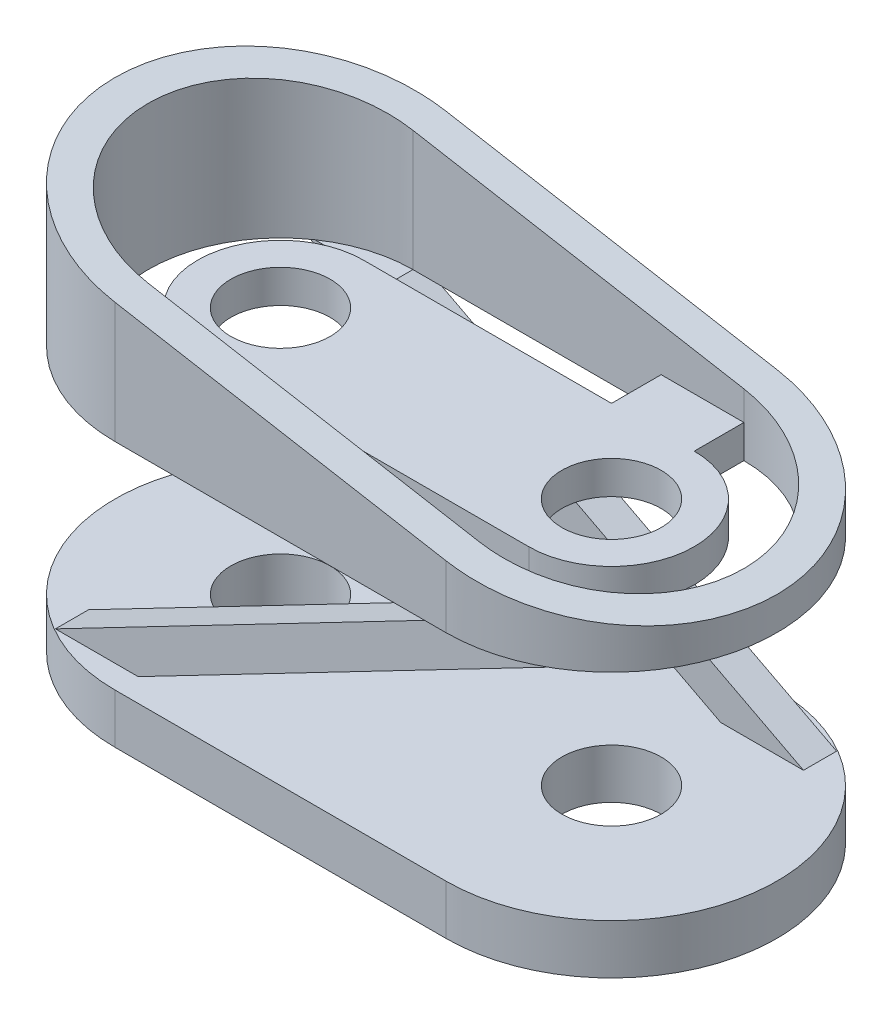
ISO-10303-21;
HEADER;
FILE_DESCRIPTION(('STEP AP214'),'2;1');
FILE_NAME('part.step','',(''),(''),'','','');
FILE_SCHEMA(('AUTOMOTIVE_DESIGN { 1 0 10303 214 1 1 1 1 }'));
ENDSEC;
DATA;
#1=APPLICATION_CONTEXT('core data for automotive mechanical design processes');
#2=APPLICATION_PROTOCOL_DEFINITION('international standard','automotive_design',2000,#1);
#3=PRODUCT_CONTEXT('',#1,'mechanical');
#4=PRODUCT('Part','Part','',(#3));
#5=PRODUCT_RELATED_PRODUCT_CATEGORY('part','',(#4));
#6=PRODUCT_DEFINITION_FORMATION('','',#4);
#7=PRODUCT_DEFINITION_CONTEXT('part definition',#1,'design');
#8=PRODUCT_DEFINITION('design','',#6,#7);
#9=PRODUCT_DEFINITION_SHAPE('','',#8);
#10=(LENGTH_UNIT() NAMED_UNIT(*) SI_UNIT(.MILLI.,.METRE.));
#11=(NAMED_UNIT(*) PLANE_ANGLE_UNIT() SI_UNIT($,.RADIAN.));
#12=(NAMED_UNIT(*) SI_UNIT($,.STERADIAN.) SOLID_ANGLE_UNIT());
#13=UNCERTAINTY_MEASURE_WITH_UNIT(LENGTH_MEASURE(1.E-05),#10,'distance_accuracy_value','');
#14=(GEOMETRIC_REPRESENTATION_CONTEXT(3) GLOBAL_UNCERTAINTY_ASSIGNED_CONTEXT((#13)) GLOBAL_UNIT_ASSIGNED_CONTEXT((#10,
#11,#12)) REPRESENTATION_CONTEXT('',''));
#15=CARTESIAN_POINT('',(0.,0.,0.));
#16=DIRECTION('',(0.,0.,1.));
#17=DIRECTION('',(1.,0.,0.));
#18=AXIS2_PLACEMENT_3D('',#15,#16,#17);
#19=CARTESIAN_POINT('',(-50.,15.,0.));
#20=DIRECTION('',(0.,1.,0.));
#21=DIRECTION('',(0.,0.,1.));
#22=AXIS2_PLACEMENT_3D('',#19,#20,#21);
#23=PLANE('',#22);
#24=CARTESIAN_POINT('',(-50.,15.,0.));
#25=DIRECTION('',(0.,1.,0.));
#26=DIRECTION('',(0.,0.,1.));
#27=AXIS2_PLACEMENT_3D('',#24,#25,#26);
#28=CIRCLE('',#27,15.);
#29=CARTESIAN_POINT('',(-50.,15.,15.));
#30=VERTEX_POINT('',#29);
#31=EDGE_CURVE('E489',#30,#30,#28,.T.);
#32=ORIENTED_EDGE('',*,*,#31,.F.);
#33=EDGE_LOOP('',(#32));
#34=FACE_BOUND('',#33,.T.);
#35=CARTESIAN_POINT('',(50.,15.,0.));
#36=DIRECTION('',(0.,1.,0.));
#37=DIRECTION('',(0.,0.,1.));
#38=AXIS2_PLACEMENT_3D('',#35,#36,#37);
#39=CIRCLE('',#38,15.);
#40=CARTESIAN_POINT('',(50.,15.,15.));
#41=VERTEX_POINT('',#40);
#42=EDGE_CURVE('E476',#41,#41,#39,.T.);
#43=ORIENTED_EDGE('',*,*,#42,.F.);
#44=EDGE_LOOP('',(#43));
#45=FACE_BOUND('',#44,.T.);
#46=CARTESIAN_POINT('',(-50.,15.,0.));
#47=DIRECTION('',(0.,1.,0.));
#48=DIRECTION('',(0.,0.,1.));
#49=AXIS2_PLACEMENT_3D('',#46,#47,#48);
#50=CIRCLE('',#49,50.);
#51=CARTESIAN_POINT('',(-50.,15.,-50.));
#52=VERTEX_POINT('',#51);
#53=CARTESIAN_POINT('',(-50.,15.,50.));
#54=VERTEX_POINT('',#53);
#55=EDGE_CURVE('E443',#52,#54,#50,.T.);
#56=ORIENTED_EDGE('',*,*,#55,.T.);
#57=DIRECTION('',(1.,0.,0.));
#58=VECTOR('',#57,1.);
#59=CARTESIAN_POINT('',(-50.,15.,50.));
#60=LINE('',#59,#58);
#61=CARTESIAN_POINT('',(50.,15.,50.));
#62=VERTEX_POINT('',#61);
#63=EDGE_CURVE('E450',#54,#62,#60,.T.);
#64=ORIENTED_EDGE('',*,*,#63,.T.);
#65=CARTESIAN_POINT('',(50.,15.,0.));
#66=DIRECTION('',(0.,1.,0.));
#67=DIRECTION('',(0.,0.,1.));
#68=AXIS2_PLACEMENT_3D('',#65,#66,#67);
#69=CIRCLE('',#68,50.);
#70=CARTESIAN_POINT('',(50.,15.,-50.));
#71=VERTEX_POINT('',#70);
#72=EDGE_CURVE('E448',#62,#71,#69,.T.);
#73=ORIENTED_EDGE('',*,*,#72,.T.);
#74=DIRECTION('',(-1.,0.,0.));
#75=VECTOR('',#74,1.);
#76=CARTESIAN_POINT('',(-50.,15.,-50.));
#77=LINE('',#76,#75);
#78=EDGE_CURVE('E455',#71,#52,#77,.T.);
#79=ORIENTED_EDGE('',*,*,#78,.T.);
#80=EDGE_LOOP('',(#56,#64,#73,#79));
#81=FACE_BOUND('',#80,.T.);
#82=DIRECTION('',(0.,0.,1.));
#83=VECTOR('',#82,1.);
#84=CARTESIAN_POINT('',(50.,15.,-43.));
#85=LINE('',#84,#83);
#86=CARTESIAN_POINT('',(50.,15.,-43.));
#87=VERTEX_POINT('',#86);
#88=CARTESIAN_POINT('',(50.,15.,-33.));
#89=VERTEX_POINT('',#88);
#90=EDGE_CURVE('E438',#87,#89,#85,.T.);
#91=ORIENTED_EDGE('',*,*,#90,.F.);
#92=DIRECTION('',(1.,0.,0.));
#93=VECTOR('',#92,1.);
#94=CARTESIAN_POINT('',(50.,15.,-43.));
#95=LINE('',#94,#93);
#96=CARTESIAN_POINT('',(75.,15.,-43.));
#97=VERTEX_POINT('',#96);
#98=EDGE_CURVE('E424',#87,#97,#95,.T.);
#99=ORIENTED_EDGE('',*,*,#98,.T.);
#100=DIRECTION('',(0.,0.,1.));
#101=VECTOR('',#100,1.);
#102=CARTESIAN_POINT('',(75.,15.,-43.));
#103=LINE('',#102,#101);
#104=CARTESIAN_POINT('',(75.,15.,-33.));
#105=VERTEX_POINT('',#104);
#106=EDGE_CURVE('E441',#97,#105,#103,.T.);
#107=ORIENTED_EDGE('',*,*,#106,.T.);
#108=DIRECTION('',(1.,0.,0.));
#109=VECTOR('',#108,1.);
#110=CARTESIAN_POINT('',(50.,15.,-33.));
#111=LINE('',#110,#109);
#112=EDGE_CURVE('E414',#89,#105,#111,.T.);
#113=ORIENTED_EDGE('',*,*,#112,.F.);
#114=EDGE_LOOP('',(#91,#99,#107,#113));
#115=FACE_BOUND('',#114,.T.);
#116=DIRECTION('',(0.,0.,-1.));
#117=VECTOR('',#116,1.);
#118=CARTESIAN_POINT('',(-50.,15.,43.));
#119=LINE('',#118,#117);
#120=CARTESIAN_POINT('',(-50.,15.,43.));
#121=VERTEX_POINT('',#120);
#122=CARTESIAN_POINT('',(-50.,15.,33.));
#123=VERTEX_POINT('',#122);
#124=EDGE_CURVE('E62',#121,#123,#119,.T.);
#125=ORIENTED_EDGE('',*,*,#124,.F.);
#126=DIRECTION('',(-1.,0.,0.));
#127=VECTOR('',#126,1.);
#128=CARTESIAN_POINT('',(-50.,15.,43.));
#129=LINE('',#128,#127);
#130=CARTESIAN_POINT('',(-75.,15.,43.));
#131=VERTEX_POINT('',#130);
#132=EDGE_CURVE('E57',#121,#131,#129,.T.);
#133=ORIENTED_EDGE('',*,*,#132,.T.);
#134=DIRECTION('',(0.,0.,-1.));
#135=VECTOR('',#134,1.);
#136=CARTESIAN_POINT('',(-75.,15.,43.));
#137=LINE('',#136,#135);
#138=CARTESIAN_POINT('',(-75.,15.,33.));
#139=VERTEX_POINT('',#138);
#140=EDGE_CURVE('E234',#131,#139,#137,.T.);
#141=ORIENTED_EDGE('',*,*,#140,.T.);
#142=DIRECTION('',(-1.,0.,0.));
#143=VECTOR('',#142,1.);
#144=CARTESIAN_POINT('',(-50.,15.,33.));
#145=LINE('',#144,#143);
#146=EDGE_CURVE('E236',#123,#139,#145,.T.);
#147=ORIENTED_EDGE('',*,*,#146,.F.);
#148=EDGE_LOOP('',(#125,#133,#141,#147));
#149=FACE_BOUND('',#148,.T.);
#150=ADVANCED_FACE('F39',(#34,#45,#81,#115,#149),#23,.T.);
#151=CARTESIAN_POINT('',(-50.,80.,0.));
#152=DIRECTION('',(0.,1.,0.));
#153=DIRECTION('',(0.,0.,1.));
#154=AXIS2_PLACEMENT_3D('',#151,#152,#153);
#155=PLANE('',#154);
#156=CARTESIAN_POINT('',(-50.,80.,0.));
#157=DIRECTION('',(0.,1.,0.));
#158=DIRECTION('',(0.,0.,1.));
#159=AXIS2_PLACEMENT_3D('',#156,#157,#158);
#160=CIRCLE('',#159,15.);
#161=CARTESIAN_POINT('',(-50.,80.,15.));
#162=VERTEX_POINT('',#161);
#163=EDGE_CURVE('E487',#162,#162,#160,.T.);
#164=ORIENTED_EDGE('',*,*,#163,.T.);
#165=EDGE_LOOP('',(#164));
#166=FACE_BOUND('',#165,.T.);
#167=CARTESIAN_POINT('',(50.,80.,0.));
#168=DIRECTION('',(0.,1.,0.));
#169=DIRECTION('',(0.,0.,1.));
#170=AXIS2_PLACEMENT_3D('',#167,#168,#169);
#171=CIRCLE('',#170,15.);
#172=CARTESIAN_POINT('',(50.,80.,15.));
#173=VERTEX_POINT('',#172);
#174=EDGE_CURVE('E471',#173,#173,#171,.T.);
#175=ORIENTED_EDGE('',*,*,#174,.T.);
#176=EDGE_LOOP('',(#175));
#177=FACE_BOUND('',#176,.T.);
#178=DIRECTION('',(-1.,0.,0.));
#179=VECTOR('',#178,1.);
#180=CARTESIAN_POINT('',(50.,80.,-50.));
#181=LINE('',#180,#179);
#182=CARTESIAN_POINT('',(50.,80.,-50.));
#183=VERTEX_POINT('',#182);
#184=CARTESIAN_POINT('',(-50.,80.,-50.));
#185=VERTEX_POINT('',#184);
#186=EDGE_CURVE('E373',#183,#185,#181,.T.);
#187=ORIENTED_EDGE('',*,*,#186,.F.);
#188=CARTESIAN_POINT('',(50.,80.,0.));
#189=DIRECTION('',(0.,1.,0.));
#190=DIRECTION('',(0.,0.,1.));
#191=AXIS2_PLACEMENT_3D('',#188,#189,#190);
#192=CIRCLE('',#191,50.);
#193=CARTESIAN_POINT('',(50.,80.,50.));
#194=VERTEX_POINT('',#193);
#195=EDGE_CURVE('E336',#194,#183,#192,.T.);
#196=ORIENTED_EDGE('',*,*,#195,.F.);
#197=DIRECTION('',(1.,0.,0.));
#198=VECTOR('',#197,1.);
#199=CARTESIAN_POINT('',(-50.,80.,50.));
#200=LINE('',#199,#198);
#201=CARTESIAN_POINT('',(-50.,80.,50.));
#202=VERTEX_POINT('',#201);
#203=EDGE_CURVE('E334',#202,#194,#200,.T.);
#204=ORIENTED_EDGE('',*,*,#203,.F.);
#205=CARTESIAN_POINT('',(-50.,80.,0.));
#206=DIRECTION('',(0.,1.,0.));
#207=DIRECTION('',(0.,0.,1.));
#208=AXIS2_PLACEMENT_3D('',#205,#206,#207);
#209=CIRCLE('',#208,50.);
#210=EDGE_CURVE('E325',#185,#202,#209,.T.);
#211=ORIENTED_EDGE('',*,*,#210,.F.);
#212=EDGE_LOOP('',(#187,#196,#204,#211));
#213=FACE_BOUND('',#212,.T.);
#214=DIRECTION('',(-1.,0.,0.));
#215=VECTOR('',#214,1.);
#216=CARTESIAN_POINT('',(-50.,80.,-33.));
#217=LINE('',#216,#215);
#218=CARTESIAN_POINT('',(-72.6053091109146,80.,-33.));
#219=VERTEX_POINT('',#218);
#220=CARTESIAN_POINT('',(-75.,80.,-33.));
#221=VERTEX_POINT('',#220);
#222=EDGE_CURVE('E417',#219,#221,#217,.T.);
#223=ORIENTED_EDGE('',*,*,#222,.F.);
#224=CARTESIAN_POINT('',(-50.,80.,0.));
#225=DIRECTION('',(0.,1.,0.));
#226=DIRECTION('',(0.,0.,1.));
#227=AXIS2_PLACEMENT_3D('',#224,#225,#226);
#228=CIRCLE('',#227,40.);
#229=CARTESIAN_POINT('',(-50.,80.,40.));
#230=VERTEX_POINT('',#229);
#231=EDGE_CURVE('E302',#219,#230,#228,.T.);
#232=ORIENTED_EDGE('',*,*,#231,.T.);
#233=DIRECTION('',(0.,0.,-1.));
#234=VECTOR('',#233,1.);
#235=CARTESIAN_POINT('',(-50.,80.,45.));
#236=LINE('',#235,#234);
#237=CARTESIAN_POINT('',(-50.,80.,25.));
#238=VERTEX_POINT('',#237);
#239=EDGE_CURVE('E273',#230,#238,#236,.T.);
#240=ORIENTED_EDGE('',*,*,#239,.T.);
#241=CARTESIAN_POINT('',(-50.,80.,0.));
#242=DIRECTION('',(0.,1.,0.));
#243=DIRECTION('',(0.,0.,1.));
#244=AXIS2_PLACEMENT_3D('',#241,#242,#243);
#245=CIRCLE('',#244,25.);
#246=CARTESIAN_POINT('',(-50.,80.,-25.));
#247=VERTEX_POINT('',#246);
#248=EDGE_CURVE('E378',#247,#238,#245,.T.);
#249=ORIENTED_EDGE('',*,*,#248,.F.);
#250=DIRECTION('',(-1.,0.,0.));
#251=VECTOR('',#250,1.);
#252=CARTESIAN_POINT('',(-50.,80.,-25.));
#253=LINE('',#252,#251);
#254=CARTESIAN_POINT('',(25.,80.,-25.));
#255=VERTEX_POINT('',#254);
#256=EDGE_CURVE('E380',#255,#247,#253,.T.);
#257=ORIENTED_EDGE('',*,*,#256,.F.);
#258=DIRECTION('',(0.,0.,1.));
#259=VECTOR('',#258,1.);
#260=CARTESIAN_POINT('',(25.,80.,-50.));
#261=LINE('',#260,#259);
#262=CARTESIAN_POINT('',(25.,80.,-40.));
#263=VERTEX_POINT('',#262);
#264=EDGE_CURVE('E374',#263,#255,#261,.T.);
#265=ORIENTED_EDGE('',*,*,#264,.F.);
#266=DIRECTION('',(-1.,0.,0.));
#267=VECTOR('',#266,1.);
#268=CARTESIAN_POINT('',(-50.,80.,-40.));
#269=LINE('',#268,#267);
#270=CARTESIAN_POINT('',(-50.,80.,-40.));
#271=VERTEX_POINT('',#270);
#272=EDGE_CURVE('E317',#263,#271,#269,.T.);
#273=ORIENTED_EDGE('',*,*,#272,.T.);
#274=DIRECTION('',(0.,0.,1.));
#275=VECTOR('',#274,1.);
#276=CARTESIAN_POINT('',(-50.,80.,-43.));
#277=LINE('',#276,#275);
#278=CARTESIAN_POINT('',(-50.,80.,-43.));
#279=VERTEX_POINT('',#278);
#280=EDGE_CURVE('E433',#279,#271,#277,.T.);
#281=ORIENTED_EDGE('',*,*,#280,.F.);
#282=DIRECTION('',(-1.,0.,0.));
#283=VECTOR('',#282,1.);
#284=CARTESIAN_POINT('',(-50.,80.,-43.));
#285=LINE('',#284,#283);
#286=CARTESIAN_POINT('',(-75.,80.,-43.));
#287=VERTEX_POINT('',#286);
#288=EDGE_CURVE('E427',#279,#287,#285,.T.);
#289=ORIENTED_EDGE('',*,*,#288,.T.);
#290=DIRECTION('',(0.,0.,1.));
#291=VECTOR('',#290,1.);
#292=CARTESIAN_POINT('',(-75.,80.,-43.));
#293=LINE('',#292,#291);
#294=EDGE_CURVE('E436',#287,#221,#293,.T.);
#295=ORIENTED_EDGE('',*,*,#294,.T.);
#296=EDGE_LOOP('',(#223,#232,#240,#249,#257,#265,#273,#281,#289,#295));
#297=FACE_BOUND('',#296,.T.);
#298=DIRECTION('',(0.,0.,-1.));
#299=VECTOR('',#298,1.);
#300=CARTESIAN_POINT('',(50.,80.,43.));
#301=LINE('',#300,#299);
#302=CARTESIAN_POINT('',(50.,80.,43.));
#303=VERTEX_POINT('',#302);
#304=CARTESIAN_POINT('',(50.,80.,40.));
#305=VERTEX_POINT('',#304);
#306=EDGE_CURVE('E267',#303,#305,#301,.T.);
#307=ORIENTED_EDGE('',*,*,#306,.F.);
#308=DIRECTION('',(1.,0.,0.));
#309=VECTOR('',#308,1.);
#310=CARTESIAN_POINT('',(50.,80.,43.));
#311=LINE('',#310,#309);
#312=CARTESIAN_POINT('',(75.,80.,43.));
#313=VERTEX_POINT('',#312);
#314=EDGE_CURVE('E257',#303,#313,#311,.T.);
#315=ORIENTED_EDGE('',*,*,#314,.T.);
#316=DIRECTION('',(0.,0.,-1.));
#317=VECTOR('',#316,1.);
#318=CARTESIAN_POINT('',(75.,80.,43.));
#319=LINE('',#318,#317);
#320=CARTESIAN_POINT('',(75.,80.,33.));
#321=VERTEX_POINT('',#320);
#322=EDGE_CURVE('E270',#313,#321,#319,.T.);
#323=ORIENTED_EDGE('',*,*,#322,.T.);
#324=DIRECTION('',(1.,0.,0.));
#325=VECTOR('',#324,1.);
#326=CARTESIAN_POINT('',(50.,80.,33.));
#327=LINE('',#326,#325);
#328=CARTESIAN_POINT('',(72.6053091109146,80.,33.));
#329=VERTEX_POINT('',#328);
#330=EDGE_CURVE('E491',#329,#321,#327,.T.);
#331=ORIENTED_EDGE('',*,*,#330,.F.);
#332=CARTESIAN_POINT('',(50.,80.,0.));
#333=DIRECTION('',(0.,1.,0.));
#334=DIRECTION('',(0.,0.,1.));
#335=AXIS2_PLACEMENT_3D('',#332,#333,#334);
#336=CIRCLE('',#335,40.);
#337=CARTESIAN_POINT('',(50.,80.,-40.));
#338=VERTEX_POINT('',#337);
#339=EDGE_CURVE('E315',#329,#338,#336,.T.);
#340=ORIENTED_EDGE('',*,*,#339,.T.);
#341=DIRECTION('',(0.,0.,-1.));
#342=VECTOR('',#341,1.);
#343=CARTESIAN_POINT('',(50.,80.,-25.));
#344=LINE('',#343,#342);
#345=CARTESIAN_POINT('',(50.,80.,-25.));
#346=VERTEX_POINT('',#345);
#347=EDGE_CURVE('E354',#346,#338,#344,.T.);
#348=ORIENTED_EDGE('',*,*,#347,.F.);
#349=CARTESIAN_POINT('',(50.,80.,0.));
#350=DIRECTION('',(0.,1.,0.));
#351=DIRECTION('',(0.,0.,1.));
#352=AXIS2_PLACEMENT_3D('',#349,#350,#351);
#353=CIRCLE('',#352,25.);
#354=CARTESIAN_POINT('',(50.,80.,25.));
#355=VERTEX_POINT('',#354);
#356=EDGE_CURVE('E359',#355,#346,#353,.T.);
#357=ORIENTED_EDGE('',*,*,#356,.F.);
#358=DIRECTION('',(1.,0.,0.));
#359=VECTOR('',#358,1.);
#360=CARTESIAN_POINT('',(-50.,80.,25.));
#361=LINE('',#360,#359);
#362=CARTESIAN_POINT('',(-25.,80.,25.));
#363=VERTEX_POINT('',#362);
#364=EDGE_CURVE('E382',#363,#355,#361,.T.);
#365=ORIENTED_EDGE('',*,*,#364,.F.);
#366=DIRECTION('',(0.,0.,-1.));
#367=VECTOR('',#366,1.);
#368=CARTESIAN_POINT('',(-25.,80.,45.));
#369=LINE('',#368,#367);
#370=CARTESIAN_POINT('',(-25.,80.,40.));
#371=VERTEX_POINT('',#370);
#372=EDGE_CURVE('E281',#371,#363,#369,.T.);
#373=ORIENTED_EDGE('',*,*,#372,.F.);
#374=DIRECTION('',(1.,0.,0.));
#375=VECTOR('',#374,1.);
#376=CARTESIAN_POINT('',(-50.,80.,40.));
#377=LINE('',#376,#375);
#378=EDGE_CURVE('E309',#371,#305,#377,.T.);
#379=ORIENTED_EDGE('',*,*,#378,.T.);
#380=EDGE_LOOP('',(#307,#315,#323,#331,#340,#348,#357,#365,#373,#379));
#381=FACE_BOUND('',#380,.T.);
#382=ADVANCED_FACE('F502',(#166,#177,#213,#297,#381),#155,.F.);
#383=CARTESIAN_POINT('',(-50.,80.,-43.));
#384=DIRECTION('',(0.,1.,0.));
#385=DIRECTION('',(-1.,0.,0.));
#386=AXIS2_PLACEMENT_3D('',#383,#384,#385);
#387=PLANE('',#386);
#388=CARTESIAN_POINT('',(-50.,80.,-33.));
#389=VERTEX_POINT('',#388);
#390=EDGE_CURVE('E435',#271,#389,#277,.T.);
#391=ORIENTED_EDGE('',*,*,#390,.F.);
#392=EDGE_CURVE('E310',#271,#219,#228,.T.);
#393=ORIENTED_EDGE('',*,*,#392,.T.);
#394=EDGE_CURVE('E418',#389,#219,#217,.T.);
#395=ORIENTED_EDGE('',*,*,#394,.F.);
#396=EDGE_LOOP('',(#391,#393,#395));
#397=FACE_BOUND('',#396,.T.);
#398=ADVANCED_FACE('F537',(#397),#387,.T.);
#399=CARTESIAN_POINT('',(-50.,15.,0.));
#400=DIRECTION('',(0.,-1.,0.));
#401=DIRECTION('',(0.,0.,-1.));
#402=AXIS2_PLACEMENT_3D('',#399,#400,#401);
#403=CYLINDRICAL_SURFACE('',#402,50.);
#404=CARTESIAN_POINT('',(-50.,0.,0.));
#405=DIRECTION('',(0.,1.,0.));
#406=DIRECTION('',(0.,0.,1.));
#407=AXIS2_PLACEMENT_3D('',#404,#405,#406);
#408=CIRCLE('',#407,50.);
#409=CARTESIAN_POINT('',(-50.,0.,-50.));
#410=VERTEX_POINT('',#409);
#411=CARTESIAN_POINT('',(-50.,0.,50.));
#412=VERTEX_POINT('',#411);
#413=EDGE_CURVE('E442',#410,#412,#408,.T.);
#414=ORIENTED_EDGE('',*,*,#413,.T.);
#415=DIRECTION('',(0.,-1.,0.));
#416=VECTOR('',#415,1.);
#417=CARTESIAN_POINT('',(-50.,15.,50.));
#418=LINE('',#417,#416);
#419=EDGE_CURVE('E11',#54,#412,#418,.T.);
#420=ORIENTED_EDGE('',*,*,#419,.F.);
#421=ORIENTED_EDGE('',*,*,#55,.F.);
#422=DIRECTION('',(0.,-1.,0.));
#423=VECTOR('',#422,1.);
#424=CARTESIAN_POINT('',(-50.,15.,-50.));
#425=LINE('',#424,#423);
#426=EDGE_CURVE('E451',#52,#410,#425,.T.);
#427=ORIENTED_EDGE('',*,*,#426,.T.);
#428=EDGE_LOOP('',(#414,#420,#421,#427));
#429=FACE_BOUND('',#428,.T.);
#430=ADVANCED_FACE('F41',(#429),#403,.T.);
#431=CARTESIAN_POINT('',(-50.,15.,50.));
#432=DIRECTION('',(0.,0.,-1.));
#433=DIRECTION('',(-1.,0.,0.));
#434=AXIS2_PLACEMENT_3D('',#431,#432,#433);
#435=PLANE('',#434);
#436=DIRECTION('',(1.,0.,0.));
#437=VECTOR('',#436,1.);
#438=CARTESIAN_POINT('',(-50.,0.,50.));
#439=LINE('',#438,#437);
#440=CARTESIAN_POINT('',(50.,0.,50.));
#441=VERTEX_POINT('',#440);
#442=EDGE_CURVE('E459',#412,#441,#439,.T.);
#443=ORIENTED_EDGE('',*,*,#442,.T.);
#444=DIRECTION('',(0.,-1.,0.));
#445=VECTOR('',#444,1.);
#446=CARTESIAN_POINT('',(50.,15.,50.));
#447=LINE('',#446,#445);
#448=EDGE_CURVE('E48',#62,#441,#447,.T.);
#449=ORIENTED_EDGE('',*,*,#448,.F.);
#450=ORIENTED_EDGE('',*,*,#63,.F.);
#451=ORIENTED_EDGE('',*,*,#419,.T.);
#452=EDGE_LOOP('',(#443,#449,#450,#451));
#453=FACE_BOUND('',#452,.T.);
#454=ADVANCED_FACE('F554',(#453),#435,.F.);
#455=CARTESIAN_POINT('',(50.,15.,0.));
#456=DIRECTION('',(0.,-1.,0.));
#457=DIRECTION('',(0.,0.,-1.));
#458=AXIS2_PLACEMENT_3D('',#455,#456,#457);
#459=CYLINDRICAL_SURFACE('',#458,50.);
#460=CARTESIAN_POINT('',(50.,0.,0.));
#461=DIRECTION('',(0.,1.,0.));
#462=DIRECTION('',(0.,0.,1.));
#463=AXIS2_PLACEMENT_3D('',#460,#461,#462);
#464=CIRCLE('',#463,50.);
#465=CARTESIAN_POINT('',(50.,0.,-50.));
#466=VERTEX_POINT('',#465);
#467=EDGE_CURVE('E456',#441,#466,#464,.T.);
#468=ORIENTED_EDGE('',*,*,#467,.T.);
#469=DIRECTION('',(0.,-1.,0.));
#470=VECTOR('',#469,1.);
#471=CARTESIAN_POINT('',(50.,15.,-50.));
#472=LINE('',#471,#470);
#473=EDGE_CURVE('E463',#71,#466,#472,.T.);
#474=ORIENTED_EDGE('',*,*,#473,.F.);
#475=ORIENTED_EDGE('',*,*,#72,.F.);
#476=ORIENTED_EDGE('',*,*,#448,.T.);
#477=EDGE_LOOP('',(#468,#474,#475,#476));
#478=FACE_BOUND('',#477,.T.);
#479=ADVANCED_FACE('F552',(#478),#459,.T.);
#480=CARTESIAN_POINT('',(-50.,15.,-50.));
#481=DIRECTION('',(0.,0.,1.));
#482=DIRECTION('',(1.,0.,0.));
#483=AXIS2_PLACEMENT_3D('',#480,#481,#482);
#484=PLANE('',#483);
#485=DIRECTION('',(-1.,0.,0.));
#486=VECTOR('',#485,1.);
#487=CARTESIAN_POINT('',(-50.,0.,-50.));
#488=LINE('',#487,#486);
#489=EDGE_CURVE('E449',#466,#410,#488,.T.);
#490=ORIENTED_EDGE('',*,*,#489,.T.);
#491=ORIENTED_EDGE('',*,*,#426,.F.);
#492=ORIENTED_EDGE('',*,*,#78,.F.);
#493=ORIENTED_EDGE('',*,*,#473,.T.);
#494=EDGE_LOOP('',(#490,#491,#492,#493));
#495=FACE_BOUND('',#494,.T.);
#496=ADVANCED_FACE('F547',(#495),#484,.F.);
#497=CARTESIAN_POINT('',(-50.,0.,0.));
#498=DIRECTION('',(0.,1.,0.));
#499=DIRECTION('',(0.,0.,1.));
#500=AXIS2_PLACEMENT_3D('',#497,#498,#499);
#501=PLANE('',#500);
#502=CARTESIAN_POINT('',(-50.,0.,0.));
#503=DIRECTION('',(0.,1.,0.));
#504=DIRECTION('',(0.,0.,1.));
#505=AXIS2_PLACEMENT_3D('',#502,#503,#504);
#506=CIRCLE('',#505,15.);
#507=CARTESIAN_POINT('',(-50.,0.,15.));
#508=VERTEX_POINT('',#507);
#509=EDGE_CURVE('E483',#508,#508,#506,.T.);
#510=ORIENTED_EDGE('',*,*,#509,.T.);
#511=EDGE_LOOP('',(#510));
#512=FACE_BOUND('',#511,.T.);
#513=CARTESIAN_POINT('',(50.,0.,0.));
#514=DIRECTION('',(0.,1.,0.));
#515=DIRECTION('',(0.,0.,1.));
#516=AXIS2_PLACEMENT_3D('',#513,#514,#515);
#517=CIRCLE('',#516,15.);
#518=CARTESIAN_POINT('',(50.,0.,15.));
#519=VERTEX_POINT('',#518);
#520=EDGE_CURVE('E468',#519,#519,#517,.T.);
#521=ORIENTED_EDGE('',*,*,#520,.T.);
#522=EDGE_LOOP('',(#521));
#523=FACE_BOUND('',#522,.T.);
#524=ORIENTED_EDGE('',*,*,#413,.F.);
#525=ORIENTED_EDGE('',*,*,#489,.F.);
#526=ORIENTED_EDGE('',*,*,#467,.F.);
#527=ORIENTED_EDGE('',*,*,#442,.F.);
#528=EDGE_LOOP('',(#524,#525,#526,#527));
#529=FACE_BOUND('',#528,.T.);
#530=ADVANCED_FACE('F543',(#512,#523,#529),#501,.F.);
#531=CARTESIAN_POINT('',(-50.,80.,-43.));
#532=DIRECTION('',(-0.461352736641989,-0.887216801234595,0.));
#533=DIRECTION('',(0.887216801234595,-0.461352736641989,0.));
#534=AXIS2_PLACEMENT_3D('',#531,#532,#533);
#535=PLANE('',#534);
#536=ORIENTED_EDGE('',*,*,#280,.T.);
#537=ORIENTED_EDGE('',*,*,#390,.T.);
#538=DIRECTION('',(0.887216801234595,-0.461352736641989,0.));
#539=VECTOR('',#538,1.);
#540=CARTESIAN_POINT('',(-50.,80.,-33.));
#541=LINE('',#540,#539);
#542=EDGE_CURVE('E406',#389,#105,#541,.T.);
#543=ORIENTED_EDGE('',*,*,#542,.T.);
#544=ORIENTED_EDGE('',*,*,#106,.F.);
#545=DIRECTION('',(0.887216801234595,-0.461352736641989,0.));
#546=VECTOR('',#545,1.);
#547=CARTESIAN_POINT('',(-50.,80.,-43.));
#548=LINE('',#547,#546);
#549=EDGE_CURVE('E422',#279,#97,#548,.T.);
#550=ORIENTED_EDGE('',*,*,#549,.F.);
#551=EDGE_LOOP('',(#536,#537,#543,#544,#550));
#552=FACE_BOUND('',#551,.T.);
#553=ADVANCED_FACE('F545',(#552),#535,.F.);
#554=CARTESIAN_POINT('',(-75.,80.,-43.));
#555=DIRECTION('',(-0.461352736641989,-0.887216801234595,0.));
#556=DIRECTION('',(0.887216801234595,-0.461352736641989,0.));
#557=AXIS2_PLACEMENT_3D('',#554,#555,#556);
#558=PLANE('',#557);
#559=ORIENTED_EDGE('',*,*,#90,.T.);
#560=DIRECTION('',(0.887216801234595,-0.461352736641989,0.));
#561=VECTOR('',#560,1.);
#562=CARTESIAN_POINT('',(-75.,80.,-33.));
#563=LINE('',#562,#561);
#564=EDGE_CURVE('E413',#221,#89,#563,.T.);
#565=ORIENTED_EDGE('',*,*,#564,.F.);
#566=ORIENTED_EDGE('',*,*,#294,.F.);
#567=DIRECTION('',(0.887216801234595,-0.461352736641989,0.));
#568=VECTOR('',#567,1.);
#569=CARTESIAN_POINT('',(-75.,80.,-43.));
#570=LINE('',#569,#568);
#571=EDGE_CURVE('E430',#287,#87,#570,.T.);
#572=ORIENTED_EDGE('',*,*,#571,.T.);
#573=EDGE_LOOP('',(#559,#565,#566,#572));
#574=FACE_BOUND('',#573,.T.);
#575=ADVANCED_FACE('F587',(#574),#558,.T.);
#576=CARTESIAN_POINT('',(0.,0.,-43.));
#577=DIRECTION('',(0.,0.,1.));
#578=DIRECTION('',(1.,0.,0.));
#579=AXIS2_PLACEMENT_3D('',#576,#577,#578);
#580=PLANE('',#579);
#581=ORIENTED_EDGE('',*,*,#549,.T.);
#582=ORIENTED_EDGE('',*,*,#98,.F.);
#583=ORIENTED_EDGE('',*,*,#571,.F.);
#584=ORIENTED_EDGE('',*,*,#288,.F.);
#585=EDGE_LOOP('',(#581,#582,#583,#584));
#586=FACE_BOUND('',#585,.T.);
#587=ADVANCED_FACE('F582',(#586),#580,.F.);
#588=CARTESIAN_POINT('',(0.,0.,-33.));
#589=DIRECTION('',(0.,0.,1.));
#590=DIRECTION('',(1.,0.,0.));
#591=AXIS2_PLACEMENT_3D('',#588,#589,#590);
#592=PLANE('',#591);
#593=ORIENTED_EDGE('',*,*,#542,.F.);
#594=ORIENTED_EDGE('',*,*,#394,.T.);
#595=ORIENTED_EDGE('',*,*,#222,.T.);
#596=ORIENTED_EDGE('',*,*,#564,.T.);
#597=ORIENTED_EDGE('',*,*,#112,.T.);
#598=EDGE_LOOP('',(#593,#594,#595,#596,#597));
#599=FACE_BOUND('',#598,.T.);
#600=ADVANCED_FACE('F595',(#599),#592,.T.);
#601=CARTESIAN_POINT('',(-50.,90.,25.));
#602=DIRECTION('',(0.,0.,-1.));
#603=DIRECTION('',(-1.,0.,0.));
#604=AXIS2_PLACEMENT_3D('',#601,#602,#603);
#605=PLANE('',#604);
#606=DIRECTION('',(0.,1.,0.));
#607=VECTOR('',#606,1.);
#608=CARTESIAN_POINT('',(-25.,90.,25.));
#609=LINE('',#608,#607);
#610=CARTESIAN_POINT('',(-25.,90.,25.));
#611=VERTEX_POINT('',#610);
#612=EDGE_CURVE('E268',#363,#611,#609,.T.);
#613=ORIENTED_EDGE('',*,*,#612,.F.);
#614=ORIENTED_EDGE('',*,*,#364,.T.);
#615=DIRECTION('',(0.,-1.,0.));
#616=VECTOR('',#615,1.);
#617=CARTESIAN_POINT('',(50.,90.,25.));
#618=LINE('',#617,#616);
#619=CARTESIAN_POINT('',(50.,90.,25.));
#620=VERTEX_POINT('',#619);
#621=EDGE_CURVE('E387',#620,#355,#618,.T.);
#622=ORIENTED_EDGE('',*,*,#621,.F.);
#623=DIRECTION('',(1.,0.,0.));
#624=VECTOR('',#623,1.);
#625=CARTESIAN_POINT('',(-50.,90.,25.));
#626=LINE('',#625,#624);
#627=EDGE_CURVE('E366',#611,#620,#626,.T.);
#628=ORIENTED_EDGE('',*,*,#627,.F.);
#629=EDGE_LOOP('',(#613,#614,#622,#628));
#630=FACE_BOUND('',#629,.T.);
#631=ADVANCED_FACE('F637',(#630),#605,.F.);
#632=CARTESIAN_POINT('',(-50.,80.,40.));
#633=DIRECTION('',(0.,0.,1.));
#634=DIRECTION('',(1.,0.,0.));
#635=AXIS2_PLACEMENT_3D('',#632,#633,#634);
#636=PLANE('',#635);
#637=DIRECTION('',(0.,-1.,0.));
#638=VECTOR('',#637,1.);
#639=CARTESIAN_POINT('',(-25.,80.,40.));
#640=LINE('',#639,#638);
#641=CARTESIAN_POINT('',(-25.,90.,40.));
#642=VERTEX_POINT('',#641);
#643=EDGE_CURVE('E407',#642,#371,#640,.T.);
#644=ORIENTED_EDGE('',*,*,#643,.F.);
#645=DIRECTION('',(1.,0.,0.));
#646=VECTOR('',#645,1.);
#647=CARTESIAN_POINT('',(-50.,90.,40.));
#648=LINE('',#647,#646);
#649=CARTESIAN_POINT('',(-50.,90.,40.));
#650=VERTEX_POINT('',#649);
#651=EDGE_CURVE('E401',#650,#642,#648,.T.);
#652=ORIENTED_EDGE('',*,*,#651,.F.);
#653=DIRECTION('',(0.,1.,0.));
#654=VECTOR('',#653,1.);
#655=CARTESIAN_POINT('',(-50.,80.,40.));
#656=LINE('',#655,#654);
#657=CARTESIAN_POINT('',(-50.,116.449047106269,40.));
#658=VERTEX_POINT('',#657);
#659=EDGE_CURVE('E319',#650,#658,#656,.T.);
#660=ORIENTED_EDGE('',*,*,#659,.T.);
#661=DIRECTION('',(0.984807753012209,-0.173648177666924,0.));
#662=VECTOR('',#661,1.);
#663=CARTESIAN_POINT('',(-43.7668458423152,115.349973853354,40.));
#664=LINE('',#663,#662);
#665=CARTESIAN_POINT('',(50.,98.8163490354229,40.));
#666=VERTEX_POINT('',#665);
#667=EDGE_CURVE('E399',#658,#666,#664,.T.);
#668=ORIENTED_EDGE('',*,*,#667,.T.);
#669=DIRECTION('',(0.,1.,0.));
#670=VECTOR('',#669,1.);
#671=CARTESIAN_POINT('',(50.,80.,40.));
#672=LINE('',#671,#670);
#673=EDGE_CURVE('E329',#305,#666,#672,.T.);
#674=ORIENTED_EDGE('',*,*,#673,.F.);
#675=ORIENTED_EDGE('',*,*,#378,.F.);
#676=EDGE_LOOP('',(#644,#652,#660,#668,#674,#675));
#677=FACE_BOUND('',#676,.T.);
#678=ADVANCED_FACE('F514',(#677),#636,.F.);
#679=CARTESIAN_POINT('',(50.,90.,-25.));
#680=DIRECTION('',(-1.,0.,0.));
#681=DIRECTION('',(0.,0.,1.));
#682=AXIS2_PLACEMENT_3D('',#679,#680,#681);
#683=PLANE('',#682);
#684=DIRECTION('',(0.,1.,0.));
#685=VECTOR('',#684,1.);
#686=CARTESIAN_POINT('',(50.,80.,-40.));
#687=LINE('',#686,#685);
#688=CARTESIAN_POINT('',(50.,90.,-40.));
#689=VERTEX_POINT('',#688);
#690=EDGE_CURVE('E324',#338,#689,#687,.T.);
#691=ORIENTED_EDGE('',*,*,#690,.T.);
#692=DIRECTION('',(0.,0.,-1.));
#693=VECTOR('',#692,1.);
#694=CARTESIAN_POINT('',(50.,90.,-25.));
#695=LINE('',#694,#693);
#696=CARTESIAN_POINT('',(50.,90.,-25.));
#697=VERTEX_POINT('',#696);
#698=EDGE_CURVE('E358',#697,#689,#695,.T.);
#699=ORIENTED_EDGE('',*,*,#698,.F.);
#700=DIRECTION('',(0.,-1.,0.));
#701=VECTOR('',#700,1.);
#702=CARTESIAN_POINT('',(50.,90.,-25.));
#703=LINE('',#702,#701);
#704=EDGE_CURVE('E369',#697,#346,#703,.T.);
#705=ORIENTED_EDGE('',*,*,#704,.T.);
#706=ORIENTED_EDGE('',*,*,#347,.T.);
#707=EDGE_LOOP('',(#691,#699,#705,#706));
#708=FACE_BOUND('',#707,.T.);
#709=ADVANCED_FACE('F627',(#708),#683,.F.);
#710=CARTESIAN_POINT('',(25.,90.,-50.));
#711=DIRECTION('',(1.,0.,0.));
#712=DIRECTION('',(0.,0.,-1.));
#713=AXIS2_PLACEMENT_3D('',#710,#711,#712);
#714=PLANE('',#713);
#715=DIRECTION('',(0.,1.,0.));
#716=VECTOR('',#715,1.);
#717=CARTESIAN_POINT('',(25.,90.,-40.));
#718=LINE('',#717,#716);
#719=CARTESIAN_POINT('',(25.,90.,-40.));
#720=VERTEX_POINT('',#719);
#721=EDGE_CURVE('E352',#263,#720,#718,.T.);
#722=ORIENTED_EDGE('',*,*,#721,.F.);
#723=ORIENTED_EDGE('',*,*,#264,.T.);
#724=DIRECTION('',(0.,-1.,0.));
#725=VECTOR('',#724,1.);
#726=CARTESIAN_POINT('',(25.,90.,-25.));
#727=LINE('',#726,#725);
#728=CARTESIAN_POINT('',(25.,90.,-25.));
#729=VERTEX_POINT('',#728);
#730=EDGE_CURVE('E393',#729,#255,#727,.T.);
#731=ORIENTED_EDGE('',*,*,#730,.F.);
#732=DIRECTION('',(0.,0.,1.));
#733=VECTOR('',#732,1.);
#734=CARTESIAN_POINT('',(25.,90.,-50.));
#735=LINE('',#734,#733);
#736=EDGE_CURVE('E360',#720,#729,#735,.T.);
#737=ORIENTED_EDGE('',*,*,#736,.F.);
#738=EDGE_LOOP('',(#722,#723,#731,#737));
#739=FACE_BOUND('',#738,.T.);
#740=ADVANCED_FACE('F617',(#739),#714,.F.);
#741=CARTESIAN_POINT('',(-50.,90.,0.));
#742=DIRECTION('',(0.,1.,0.));
#743=DIRECTION('',(0.,0.,1.));
#744=AXIS2_PLACEMENT_3D('',#741,#742,#743);
#745=PLANE('',#744);
#746=CARTESIAN_POINT('',(-50.,90.,0.));
#747=DIRECTION('',(0.,1.,0.));
#748=DIRECTION('',(0.,0.,1.));
#749=AXIS2_PLACEMENT_3D('',#746,#747,#748);
#750=CIRCLE('',#749,15.);
#751=CARTESIAN_POINT('',(-50.,90.,15.));
#752=VERTEX_POINT('',#751);
#753=EDGE_CURVE('E43',#752,#752,#750,.T.);
#754=ORIENTED_EDGE('',*,*,#753,.F.);
#755=EDGE_LOOP('',(#754));
#756=FACE_BOUND('',#755,.T.);
#757=CARTESIAN_POINT('',(50.,90.,0.));
#758=DIRECTION('',(0.,1.,0.));
#759=DIRECTION('',(0.,0.,1.));
#760=AXIS2_PLACEMENT_3D('',#757,#758,#759);
#761=CIRCLE('',#760,15.);
#762=CARTESIAN_POINT('',(50.,90.,15.));
#763=VERTEX_POINT('',#762);
#764=EDGE_CURVE('E466',#763,#763,#761,.T.);
#765=ORIENTED_EDGE('',*,*,#764,.F.);
#766=EDGE_LOOP('',(#765));
#767=FACE_BOUND('',#766,.T.);
#768=ORIENTED_EDGE('',*,*,#698,.T.);
#769=DIRECTION('',(-1.,0.,0.));
#770=VECTOR('',#769,1.);
#771=CARTESIAN_POINT('',(-50.,90.,-40.));
#772=LINE('',#771,#770);
#773=EDGE_CURVE('E343',#689,#720,#772,.T.);
#774=ORIENTED_EDGE('',*,*,#773,.T.);
#775=ORIENTED_EDGE('',*,*,#736,.T.);
#776=DIRECTION('',(-1.,0.,0.));
#777=VECTOR('',#776,1.);
#778=CARTESIAN_POINT('',(-50.,90.,-25.));
#779=LINE('',#778,#777);
#780=CARTESIAN_POINT('',(-50.,90.,-25.));
#781=VERTEX_POINT('',#780);
#782=EDGE_CURVE('E365',#729,#781,#779,.T.);
#783=ORIENTED_EDGE('',*,*,#782,.T.);
#784=CARTESIAN_POINT('',(-50.,90.,0.));
#785=DIRECTION('',(0.,1.,0.));
#786=DIRECTION('',(0.,0.,1.));
#787=AXIS2_PLACEMENT_3D('',#784,#785,#786);
#788=CIRCLE('',#787,25.);
#789=CARTESIAN_POINT('',(-50.,90.,25.));
#790=VERTEX_POINT('',#789);
#791=EDGE_CURVE('E364',#781,#790,#788,.T.);
#792=ORIENTED_EDGE('',*,*,#791,.T.);
#793=DIRECTION('',(0.,0.,-1.));
#794=VECTOR('',#793,1.);
#795=CARTESIAN_POINT('',(-50.,90.,45.));
#796=LINE('',#795,#794);
#797=EDGE_CURVE('E279',#650,#790,#796,.T.);
#798=ORIENTED_EDGE('',*,*,#797,.F.);
#799=ORIENTED_EDGE('',*,*,#651,.T.);
#800=DIRECTION('',(0.,0.,-1.));
#801=VECTOR('',#800,1.);
#802=CARTESIAN_POINT('',(-25.,90.,45.));
#803=LINE('',#802,#801);
#804=EDGE_CURVE('E282',#642,#611,#803,.T.);
#805=ORIENTED_EDGE('',*,*,#804,.T.);
#806=ORIENTED_EDGE('',*,*,#627,.T.);
#807=CARTESIAN_POINT('',(50.,90.,0.));
#808=DIRECTION('',(0.,1.,0.));
#809=DIRECTION('',(0.,0.,1.));
#810=AXIS2_PLACEMENT_3D('',#807,#808,#809);
#811=CIRCLE('',#810,25.);
#812=EDGE_CURVE('E368',#620,#697,#811,.T.);
#813=ORIENTED_EDGE('',*,*,#812,.T.);
#814=EDGE_LOOP('',(#768,#774,#775,#783,#792,#798,#799,#805,#806,#813));
#815=FACE_BOUND('',#814,.T.);
#816=ADVANCED_FACE('F624',(#756,#767,#815),#745,.T.);
#817=CARTESIAN_POINT('',(50.,90.,-50.));
#818=DIRECTION('',(0.,0.,1.));
#819=DIRECTION('',(1.,0.,0.));
#820=AXIS2_PLACEMENT_3D('',#817,#818,#819);
#821=PLANE('',#820);
#822=DIRECTION('',(0.,1.,0.));
#823=VECTOR('',#822,1.);
#824=CARTESIAN_POINT('',(-50.,80.,-50.));
#825=LINE('',#824,#823);
#826=CARTESIAN_POINT('',(-50.,116.449047106269,-50.));
#827=VERTEX_POINT('',#826);
#828=EDGE_CURVE('E345',#185,#827,#825,.T.);
#829=ORIENTED_EDGE('',*,*,#828,.T.);
#830=DIRECTION('',(0.984807753012209,-0.173648177666924,0.));
#831=VECTOR('',#830,1.);
#832=CARTESIAN_POINT('',(51.5076844803522,98.5505035831414,-50.));
#833=LINE('',#832,#831);
#834=CARTESIAN_POINT('',(50.,98.8163490354229,-50.));
#835=VERTEX_POINT('',#834);
#836=EDGE_CURVE('E301',#827,#835,#833,.T.);
#837=ORIENTED_EDGE('',*,*,#836,.T.);
#838=DIRECTION('',(0.,-1.,0.));
#839=VECTOR('',#838,1.);
#840=CARTESIAN_POINT('',(50.,90.,-50.));
#841=LINE('',#840,#839);
#842=EDGE_CURVE('E397',#835,#183,#841,.T.);
#843=ORIENTED_EDGE('',*,*,#842,.T.);
#844=ORIENTED_EDGE('',*,*,#186,.T.);
#845=EDGE_LOOP('',(#829,#837,#843,#844));
#846=FACE_BOUND('',#845,.T.);
#847=ADVANCED_FACE('F657',(#846),#821,.F.);
#848=CARTESIAN_POINT('',(-50.,90.,-25.));
#849=DIRECTION('',(0.,0.,1.));
#850=DIRECTION('',(1.,0.,0.));
#851=AXIS2_PLACEMENT_3D('',#848,#849,#850);
#852=PLANE('',#851);
#853=ORIENTED_EDGE('',*,*,#256,.T.);
#854=DIRECTION('',(0.,-1.,0.));
#855=VECTOR('',#854,1.);
#856=CARTESIAN_POINT('',(-50.,90.,-25.));
#857=LINE('',#856,#855);
#858=EDGE_CURVE('E394',#781,#247,#857,.T.);
#859=ORIENTED_EDGE('',*,*,#858,.F.);
#860=ORIENTED_EDGE('',*,*,#782,.F.);
#861=ORIENTED_EDGE('',*,*,#730,.T.);
#862=EDGE_LOOP('',(#853,#859,#860,#861));
#863=FACE_BOUND('',#862,.T.);
#864=ADVANCED_FACE('F615',(#863),#852,.F.);
#865=CARTESIAN_POINT('',(-50.,90.,0.));
#866=DIRECTION('',(0.,-1.,0.));
#867=DIRECTION('',(0.,0.,-1.));
#868=AXIS2_PLACEMENT_3D('',#865,#866,#867);
#869=CYLINDRICAL_SURFACE('',#868,25.);
#870=ORIENTED_EDGE('',*,*,#248,.T.);
#871=DIRECTION('',(0.,-1.,0.));
#872=VECTOR('',#871,1.);
#873=CARTESIAN_POINT('',(-50.,90.,25.));
#874=LINE('',#873,#872);
#875=EDGE_CURVE('E386',#790,#238,#874,.T.);
#876=ORIENTED_EDGE('',*,*,#875,.F.);
#877=ORIENTED_EDGE('',*,*,#791,.F.);
#878=ORIENTED_EDGE('',*,*,#858,.T.);
#879=EDGE_LOOP('',(#870,#876,#877,#878));
#880=FACE_BOUND('',#879,.T.);
#881=ADVANCED_FACE('F610',(#880),#869,.T.);
#882=CARTESIAN_POINT('',(50.,90.,0.));
#883=DIRECTION('',(0.,-1.,0.));
#884=DIRECTION('',(0.,0.,-1.));
#885=AXIS2_PLACEMENT_3D('',#882,#883,#884);
#886=CYLINDRICAL_SURFACE('',#885,25.);
#887=ORIENTED_EDGE('',*,*,#356,.T.);
#888=ORIENTED_EDGE('',*,*,#704,.F.);
#889=ORIENTED_EDGE('',*,*,#812,.F.);
#890=ORIENTED_EDGE('',*,*,#621,.T.);
#891=EDGE_LOOP('',(#887,#888,#889,#890));
#892=FACE_BOUND('',#891,.T.);
#893=ADVANCED_FACE('F645',(#892),#886,.T.);
#894=CARTESIAN_POINT('',(-50.,80.,-40.));
#895=DIRECTION('',(0.,0.,-1.));
#896=DIRECTION('',(-1.,0.,0.));
#897=AXIS2_PLACEMENT_3D('',#894,#895,#896);
#898=PLANE('',#897);
#899=CARTESIAN_POINT('',(50.,98.8163490354229,-40.));
#900=VERTEX_POINT('',#899);
#901=EDGE_CURVE('E327',#689,#900,#687,.T.);
#902=ORIENTED_EDGE('',*,*,#901,.T.);
#903=DIRECTION('',(-0.984807753012209,0.173648177666924,0.));
#904=VECTOR('',#903,1.);
#905=CARTESIAN_POINT('',(-43.7668458423152,115.349973853354,-40.));
#906=LINE('',#905,#904);
#907=CARTESIAN_POINT('',(-50.,116.449047106269,-40.));
#908=VERTEX_POINT('',#907);
#909=EDGE_CURVE('E291',#900,#908,#906,.T.);
#910=ORIENTED_EDGE('',*,*,#909,.T.);
#911=DIRECTION('',(0.,1.,0.));
#912=VECTOR('',#911,1.);
#913=CARTESIAN_POINT('',(-50.,80.,-40.));
#914=LINE('',#913,#912);
#915=EDGE_CURVE('E316',#271,#908,#914,.T.);
#916=ORIENTED_EDGE('',*,*,#915,.F.);
#917=ORIENTED_EDGE('',*,*,#272,.F.);
#918=ORIENTED_EDGE('',*,*,#721,.T.);
#919=ORIENTED_EDGE('',*,*,#773,.F.);
#920=EDGE_LOOP('',(#902,#910,#916,#917,#918,#919));
#921=FACE_BOUND('',#920,.T.);
#922=ADVANCED_FACE('F623',(#921),#898,.F.);
#923=CARTESIAN_POINT('',(-50.,80.,0.));
#924=DIRECTION('',(0.,1.,0.));
#925=DIRECTION('',(0.,0.,1.));
#926=AXIS2_PLACEMENT_3D('',#923,#924,#925);
#927=CYLINDRICAL_SURFACE('',#926,50.);
#928=DIRECTION('',(0.,1.,0.));
#929=VECTOR('',#928,1.);
#930=CARTESIAN_POINT('',(-50.,80.,50.));
#931=LINE('',#930,#929);
#932=CARTESIAN_POINT('',(-50.,116.449047106269,50.));
#933=VERTEX_POINT('',#932);
#934=EDGE_CURVE('E342',#202,#933,#931,.T.);
#935=ORIENTED_EDGE('',*,*,#934,.T.);
#936=CARTESIAN_POINT('',(-50.,116.449047106269,0.));
#937=DIRECTION('',(-0.173648177666924,-0.984807753012209,0.));
#938=DIRECTION('',(-0.984807753012209,0.173648177666924,0.));
#939=AXIS2_PLACEMENT_3D('',#936,#937,#938);
#940=ELLIPSE('',#939,50.7713305942872,50.);
#941=EDGE_CURVE('E305',#827,#933,#940,.F.);
#942=ORIENTED_EDGE('',*,*,#941,.F.);
#943=ORIENTED_EDGE('',*,*,#828,.F.);
#944=ORIENTED_EDGE('',*,*,#210,.T.);
#945=EDGE_LOOP('',(#935,#942,#943,#944));
#946=FACE_BOUND('',#945,.T.);
#947=ADVANCED_FACE('F646',(#946),#927,.T.);
#948=CARTESIAN_POINT('',(50.,80.,0.));
#949=DIRECTION('',(0.,1.,0.));
#950=DIRECTION('',(0.,0.,1.));
#951=AXIS2_PLACEMENT_3D('',#948,#949,#950);
#952=CYLINDRICAL_SURFACE('',#951,50.);
#953=CARTESIAN_POINT('',(50.,98.8163490354229,0.));
#954=DIRECTION('',(-0.173648177666924,-0.984807753012209,0.));
#955=DIRECTION('',(-0.984807753012209,0.173648177666924,0.));
#956=AXIS2_PLACEMENT_3D('',#953,#954,#955);
#957=ELLIPSE('',#956,50.7713305942872,50.);
#958=CARTESIAN_POINT('',(50.,98.8163490354229,50.));
#959=VERTEX_POINT('',#958);
#960=EDGE_CURVE('E299',#959,#835,#957,.F.);
#961=ORIENTED_EDGE('',*,*,#960,.F.);
#962=DIRECTION('',(0.,1.,0.));
#963=VECTOR('',#962,1.);
#964=CARTESIAN_POINT('',(50.,80.,50.));
#965=LINE('',#964,#963);
#966=EDGE_CURVE('E347',#194,#959,#965,.T.);
#967=ORIENTED_EDGE('',*,*,#966,.F.);
#968=ORIENTED_EDGE('',*,*,#195,.T.);
#969=ORIENTED_EDGE('',*,*,#842,.F.);
#970=EDGE_LOOP('',(#961,#967,#968,#969));
#971=FACE_BOUND('',#970,.T.);
#972=ADVANCED_FACE('F778',(#971),#952,.T.);
#973=CARTESIAN_POINT('',(-50.,80.,50.));
#974=DIRECTION('',(0.,0.,1.));
#975=DIRECTION('',(1.,0.,0.));
#976=AXIS2_PLACEMENT_3D('',#973,#974,#975);
#977=PLANE('',#976);
#978=DIRECTION('',(0.984807753012209,-0.173648177666924,0.));
#979=VECTOR('',#978,1.);
#980=CARTESIAN_POINT('',(-43.7668458423152,115.349973853354,50.));
#981=LINE('',#980,#979);
#982=EDGE_CURVE('E298',#933,#959,#981,.T.);
#983=ORIENTED_EDGE('',*,*,#982,.F.);
#984=ORIENTED_EDGE('',*,*,#934,.F.);
#985=ORIENTED_EDGE('',*,*,#203,.T.);
#986=ORIENTED_EDGE('',*,*,#966,.T.);
#987=EDGE_LOOP('',(#983,#984,#985,#986));
#988=FACE_BOUND('',#987,.T.);
#989=ADVANCED_FACE('F789',(#988),#977,.T.);
#990=CARTESIAN_POINT('',(-50.,80.,0.));
#991=DIRECTION('',(0.,1.,0.));
#992=DIRECTION('',(0.,0.,1.));
#993=AXIS2_PLACEMENT_3D('',#990,#991,#992);
#994=CYLINDRICAL_SURFACE('',#993,40.);
#995=ORIENTED_EDGE('',*,*,#915,.T.);
#996=CARTESIAN_POINT('',(-50.,116.449047106269,0.));
#997=DIRECTION('',(-0.173648177666924,-0.984807753012209,0.));
#998=DIRECTION('',(-0.984807753012209,0.173648177666924,0.));
#999=AXIS2_PLACEMENT_3D('',#996,#997,#998);
#1000=ELLIPSE('',#999,40.6170644754297,40.);
#1001=EDGE_CURVE('E289',#908,#658,#1000,.F.);
#1002=ORIENTED_EDGE('',*,*,#1001,.T.);
#1003=ORIENTED_EDGE('',*,*,#659,.F.);
#1004=EDGE_CURVE('E328',#230,#650,#656,.T.);
#1005=ORIENTED_EDGE('',*,*,#1004,.F.);
#1006=ORIENTED_EDGE('',*,*,#231,.F.);
#1007=ORIENTED_EDGE('',*,*,#392,.F.);
#1008=EDGE_LOOP('',(#995,#1002,#1003,#1005,#1006,#1007));
#1009=FACE_BOUND('',#1008,.T.);
#1010=ADVANCED_FACE('F596',(#1009),#994,.F.);
#1011=CARTESIAN_POINT('',(50.,80.,0.));
#1012=DIRECTION('',(0.,1.,0.));
#1013=DIRECTION('',(0.,0.,1.));
#1014=AXIS2_PLACEMENT_3D('',#1011,#1012,#1013);
#1015=CYLINDRICAL_SURFACE('',#1014,40.);
#1016=ORIENTED_EDGE('',*,*,#673,.T.);
#1017=CARTESIAN_POINT('',(50.,98.8163490354229,0.));
#1018=DIRECTION('',(-0.173648177666924,-0.984807753012209,0.));
#1019=DIRECTION('',(-0.984807753012209,0.173648177666924,0.));
#1020=AXIS2_PLACEMENT_3D('',#1017,#1018,#1019);
#1021=ELLIPSE('',#1020,40.6170644754297,40.);
#1022=EDGE_CURVE('E290',#666,#900,#1021,.F.);
#1023=ORIENTED_EDGE('',*,*,#1022,.T.);
#1024=ORIENTED_EDGE('',*,*,#901,.F.);
#1025=ORIENTED_EDGE('',*,*,#690,.F.);
#1026=ORIENTED_EDGE('',*,*,#339,.F.);
#1027=EDGE_CURVE('E312',#305,#329,#336,.T.);
#1028=ORIENTED_EDGE('',*,*,#1027,.F.);
#1029=EDGE_LOOP('',(#1016,#1023,#1024,#1025,#1026,#1028));
#1030=FACE_BOUND('',#1029,.T.);
#1031=ADVANCED_FACE('F509',(#1030),#1015,.F.);
#1032=CARTESIAN_POINT('',(100.,90.,-110.));
#1033=DIRECTION('',(-0.173648177666924,-0.984807753012209,0.));
#1034=DIRECTION('',(0.984807753012209,-0.173648177666924,0.));
#1035=AXIS2_PLACEMENT_3D('',#1032,#1033,#1034);
#1036=PLANE('',#1035);
#1037=ORIENTED_EDGE('',*,*,#941,.T.);
#1038=ORIENTED_EDGE('',*,*,#982,.T.);
#1039=ORIENTED_EDGE('',*,*,#960,.T.);
#1040=ORIENTED_EDGE('',*,*,#836,.F.);
#1041=EDGE_LOOP('',(#1037,#1038,#1039,#1040));
#1042=FACE_BOUND('',#1041,.T.);
#1043=ORIENTED_EDGE('',*,*,#1022,.F.);
#1044=ORIENTED_EDGE('',*,*,#667,.F.);
#1045=ORIENTED_EDGE('',*,*,#1001,.F.);
#1046=ORIENTED_EDGE('',*,*,#909,.F.);
#1047=EDGE_LOOP('',(#1043,#1044,#1045,#1046));
#1048=FACE_BOUND('',#1047,.T.);
#1049=ADVANCED_FACE('F635',(#1042,#1048),#1036,.F.);
#1050=CARTESIAN_POINT('',(-25.,90.,45.));
#1051=DIRECTION('',(-1.,0.,0.));
#1052=DIRECTION('',(0.,0.,1.));
#1053=AXIS2_PLACEMENT_3D('',#1050,#1051,#1052);
#1054=PLANE('',#1053);
#1055=ORIENTED_EDGE('',*,*,#804,.F.);
#1056=ORIENTED_EDGE('',*,*,#643,.T.);
#1057=ORIENTED_EDGE('',*,*,#372,.T.);
#1058=ORIENTED_EDGE('',*,*,#612,.T.);
#1059=EDGE_LOOP('',(#1055,#1056,#1057,#1058));
#1060=FACE_BOUND('',#1059,.T.);
#1061=ADVANCED_FACE('F523',(#1060),#1054,.F.);
#1062=CARTESIAN_POINT('',(-50.,80.,45.));
#1063=DIRECTION('',(1.,0.,0.));
#1064=DIRECTION('',(0.,0.,-1.));
#1065=AXIS2_PLACEMENT_3D('',#1062,#1063,#1064);
#1066=PLANE('',#1065);
#1067=ORIENTED_EDGE('',*,*,#239,.F.);
#1068=ORIENTED_EDGE('',*,*,#1004,.T.);
#1069=ORIENTED_EDGE('',*,*,#797,.T.);
#1070=ORIENTED_EDGE('',*,*,#875,.T.);
#1071=EDGE_LOOP('',(#1067,#1068,#1069,#1070));
#1072=FACE_BOUND('',#1071,.T.);
#1073=ADVANCED_FACE('F520',(#1072),#1066,.F.);
#1074=CARTESIAN_POINT('',(50.,80.,43.));
#1075=DIRECTION('',(0.,1.,0.));
#1076=DIRECTION('',(0.,0.,1.));
#1077=AXIS2_PLACEMENT_3D('',#1074,#1075,#1076);
#1078=PLANE('',#1077);
#1079=ORIENTED_EDGE('',*,*,#1027,.T.);
#1080=CARTESIAN_POINT('',(50.,80.,33.));
#1081=VERTEX_POINT('',#1080);
#1082=EDGE_CURVE('E494',#1081,#329,#327,.T.);
#1083=ORIENTED_EDGE('',*,*,#1082,.F.);
#1084=EDGE_CURVE('E239',#305,#1081,#301,.T.);
#1085=ORIENTED_EDGE('',*,*,#1084,.F.);
#1086=EDGE_LOOP('',(#1079,#1083,#1085));
#1087=FACE_BOUND('',#1086,.T.);
#1088=ADVANCED_FACE('F513',(#1087),#1078,.T.);
#1089=CARTESIAN_POINT('',(50.,80.,43.));
#1090=DIRECTION('',(0.461352736641989,-0.887216801234595,0.));
#1091=DIRECTION('',(0.887216801234595,0.461352736641989,0.));
#1092=AXIS2_PLACEMENT_3D('',#1089,#1090,#1091);
#1093=PLANE('',#1092);
#1094=ORIENTED_EDGE('',*,*,#306,.T.);
#1095=ORIENTED_EDGE('',*,*,#1084,.T.);
#1096=DIRECTION('',(-0.887216801234595,-0.461352736641989,0.));
#1097=VECTOR('',#1096,1.);
#1098=CARTESIAN_POINT('',(50.,80.,33.));
#1099=LINE('',#1098,#1097);
#1100=EDGE_CURVE('E250',#1081,#139,#1099,.T.);
#1101=ORIENTED_EDGE('',*,*,#1100,.T.);
#1102=ORIENTED_EDGE('',*,*,#140,.F.);
#1103=DIRECTION('',(-0.887216801234595,-0.461352736641989,0.));
#1104=VECTOR('',#1103,1.);
#1105=CARTESIAN_POINT('',(50.,80.,43.));
#1106=LINE('',#1105,#1104);
#1107=EDGE_CURVE('E263',#303,#131,#1106,.T.);
#1108=ORIENTED_EDGE('',*,*,#1107,.F.);
#1109=EDGE_LOOP('',(#1094,#1095,#1101,#1102,#1108));
#1110=FACE_BOUND('',#1109,.T.);
#1111=ADVANCED_FACE('F254',(#1110),#1093,.F.);
#1112=CARTESIAN_POINT('',(75.,80.,43.));
#1113=DIRECTION('',(0.46135273664199,-0.887216801234595,0.));
#1114=DIRECTION('',(0.887216801234595,0.46135273664199,0.));
#1115=AXIS2_PLACEMENT_3D('',#1112,#1113,#1114);
#1116=PLANE('',#1115);
#1117=ORIENTED_EDGE('',*,*,#124,.T.);
#1118=DIRECTION('',(-0.887216801234595,-0.46135273664199,0.));
#1119=VECTOR('',#1118,1.);
#1120=CARTESIAN_POINT('',(75.,80.,33.));
#1121=LINE('',#1120,#1119);
#1122=EDGE_CURVE('E249',#321,#123,#1121,.T.);
#1123=ORIENTED_EDGE('',*,*,#1122,.F.);
#1124=ORIENTED_EDGE('',*,*,#322,.F.);
#1125=DIRECTION('',(-0.887216801234595,-0.46135273664199,0.));
#1126=VECTOR('',#1125,1.);
#1127=CARTESIAN_POINT('',(75.,80.,43.));
#1128=LINE('',#1127,#1126);
#1129=EDGE_CURVE('E259',#313,#121,#1128,.T.);
#1130=ORIENTED_EDGE('',*,*,#1129,.T.);
#1131=EDGE_LOOP('',(#1117,#1123,#1124,#1130));
#1132=FACE_BOUND('',#1131,.T.);
#1133=ADVANCED_FACE('F497',(#1132),#1116,.T.);
#1134=CARTESIAN_POINT('',(0.,0.,43.));
#1135=DIRECTION('',(0.,0.,-1.));
#1136=DIRECTION('',(-1.,0.,0.));
#1137=AXIS2_PLACEMENT_3D('',#1134,#1135,#1136);
#1138=PLANE('',#1137);
#1139=ORIENTED_EDGE('',*,*,#314,.F.);
#1140=ORIENTED_EDGE('',*,*,#1107,.T.);
#1141=ORIENTED_EDGE('',*,*,#132,.F.);
#1142=ORIENTED_EDGE('',*,*,#1129,.F.);
#1143=EDGE_LOOP('',(#1139,#1140,#1141,#1142));
#1144=FACE_BOUND('',#1143,.T.);
#1145=ADVANCED_FACE('F503',(#1144),#1138,.F.);
#1146=CARTESIAN_POINT('',(0.,0.,33.));
#1147=DIRECTION('',(0.,0.,-1.));
#1148=DIRECTION('',(-1.,0.,0.));
#1149=AXIS2_PLACEMENT_3D('',#1146,#1147,#1148);
#1150=PLANE('',#1149);
#1151=ORIENTED_EDGE('',*,*,#1082,.T.);
#1152=ORIENTED_EDGE('',*,*,#330,.T.);
#1153=ORIENTED_EDGE('',*,*,#1122,.T.);
#1154=ORIENTED_EDGE('',*,*,#146,.T.);
#1155=ORIENTED_EDGE('',*,*,#1100,.F.);
#1156=EDGE_LOOP('',(#1151,#1152,#1153,#1154,#1155));
#1157=FACE_BOUND('',#1156,.T.);
#1158=ADVANCED_FACE('F246',(#1157),#1150,.T.);
#1159=CARTESIAN_POINT('',(50.,-118.5,0.));
#1160=DIRECTION('',(0.,1.,0.));
#1161=DIRECTION('',(0.,0.,1.));
#1162=AXIS2_PLACEMENT_3D('',#1159,#1160,#1161);
#1163=CYLINDRICAL_SURFACE('',#1162,15.);
#1164=ORIENTED_EDGE('',*,*,#764,.T.);
#1165=EDGE_LOOP('',(#1164));
#1166=FACE_BOUND('',#1165,.T.);
#1167=ORIENTED_EDGE('',*,*,#174,.F.);
#1168=EDGE_LOOP('',(#1167));
#1169=FACE_BOUND('',#1168,.T.);
#1170=ADVANCED_FACE('F892',(#1166,#1169),#1163,.F.);
#1171=CARTESIAN_POINT('',(-50.,-118.5,0.));
#1172=DIRECTION('',(0.,1.,0.));
#1173=DIRECTION('',(0.,0.,1.));
#1174=AXIS2_PLACEMENT_3D('',#1171,#1172,#1173);
#1175=CYLINDRICAL_SURFACE('',#1174,15.);
#1176=ORIENTED_EDGE('',*,*,#753,.T.);
#1177=EDGE_LOOP('',(#1176));
#1178=FACE_BOUND('',#1177,.T.);
#1179=ORIENTED_EDGE('',*,*,#163,.F.);
#1180=EDGE_LOOP('',(#1179));
#1181=FACE_BOUND('',#1180,.T.);
#1182=ADVANCED_FACE('F902',(#1178,#1181),#1175,.F.);
#1183=ORIENTED_EDGE('',*,*,#42,.T.);
#1184=EDGE_LOOP('',(#1183));
#1185=FACE_BOUND('',#1184,.T.);
#1186=ORIENTED_EDGE('',*,*,#520,.F.);
#1187=EDGE_LOOP('',(#1186));
#1188=FACE_BOUND('',#1187,.T.);
#1189=ADVANCED_FACE('F904',(#1185,#1188),#1163,.F.);
#1190=ORIENTED_EDGE('',*,*,#31,.T.);
#1191=EDGE_LOOP('',(#1190));
#1192=FACE_BOUND('',#1191,.T.);
#1193=ORIENTED_EDGE('',*,*,#509,.F.);
#1194=EDGE_LOOP('',(#1193));
#1195=FACE_BOUND('',#1194,.T.);
#1196=ADVANCED_FACE('F914',(#1192,#1195),#1175,.F.);
#1197=CLOSED_SHELL('',(#150,#382,#398,#430,#454,#479,#496,#530,#553,#575,#587,#600,#631,#678,
#709,#740,#816,#847,#864,#881,#893,#922,#947,#972,#989,#1010,#1031,#1049,#1061,#1073,#1088,
#1111,#1133,#1145,#1158,#1170,#1182,#1189,#1196));
#1198=MANIFOLD_SOLID_BREP('B2',#1197);
#1199=ADVANCED_BREP_SHAPE_REPRESENTATION('',(#18,#1198),#14);
#1200=SHAPE_DEFINITION_REPRESENTATION(#9,#1199);
ENDSEC;
END-ISO-10303-21;
